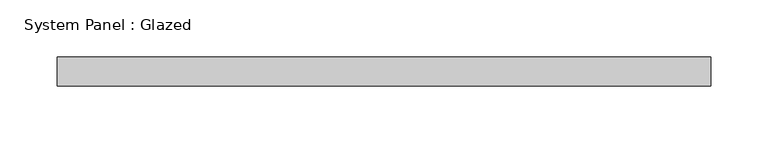
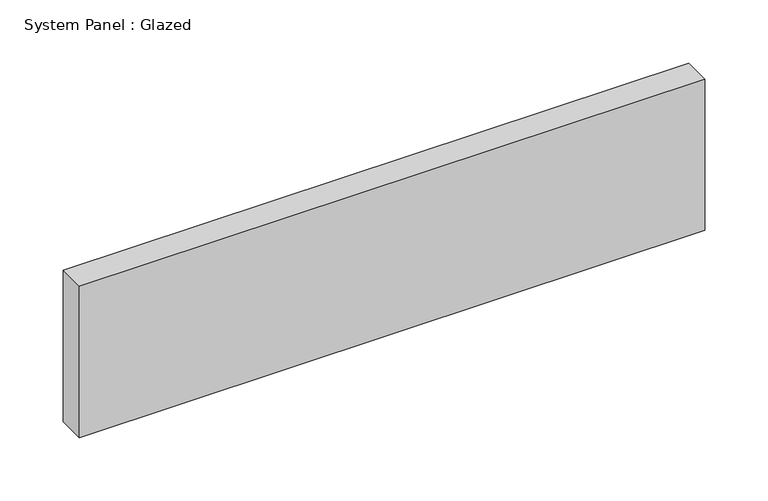
"""IFC4 building model written with IfcOpenShell, lengths in millimetres: plate geometry, System Panel : Glazed."""

from ifc_helpers import new_model, si_unit, origin, origin_with_axes, place, context, project, spatial, polyline, outline, extrude, source, transform, mapped, element, save


def system_panel_glazed_a39216e9(model_context):
    return source(origin(), model_context, "Body", "SweptSolid", [
        extrude(outline(polyline([(285.75, 19.05), (-285.75, 19.05), (-285.75, 44.45), (285.75, 44.45), (285.75, 19.05)])), origin_with_axes(), (0.0, 0.0, 1.0), 146.05),
    ])


if __name__ == "__main__":
    model = new_model("IFC4")
    model_context = context("Model", 3, world=origin())
    ifc_project = project(units=[si_unit("LENGTHUNIT", "METRE", prefix="MILLI")], contexts=[model_context])
    site = spatial("IfcSite", under=ifc_project)
    building = spatial("IfcBuilding", under=site)
    placement = place(None, origin())
    system_panel_glazed_shape = system_panel_glazed_a39216e9(model_context)
    element("IfcPlate", 1, ObjectType="System Panel : Glazed", at=placement, inside=building, context=model_context, shape_type="MappedRepresentation", body=[
        mapped(system_panel_glazed_shape, transform((0.0, 0.0, 0.0), x_axis=(1.0, 0.0, 0.0), y_axis=(0.0, 1.0, 0.0), z_axis=(0.0, 0.0, 1.0))),
    ])
    save(model, "model.ifc")

# Revit data of these elements
# Type "System Panel : Glazed"
#   Construction Type Id = "GSP4R"
#   Analytic Construction = "1/8 in Pilkington single glazing"
#   Visual Light Transmittance = 0.9
#   Solar Heat Gain Coefficient = 0.86
#   Heat Transfer Coefficient (U) = 1.18115 BTU/(h·ft²·°F)
#   Define Thermal Properties by = 1
# Element 1 (IfcPlate, "System Panel : Glazed")
#   Materials on its faces: "Glass"
# Materials
#   "Glass": class "Glass", colour RGB 0 128 192, transparency 0.75, Description = "Soda Lime Glass", Cost = 0
